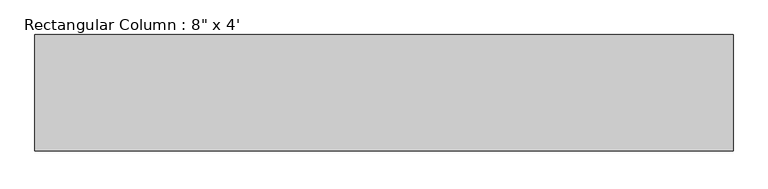
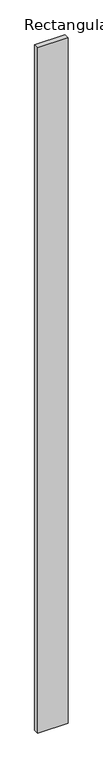
"""IFC4 building model written with IfcOpenShell, lengths in millimetres: column geometry."""

from ifc_helpers import new_model, si_unit, origin, origin_with_axes, place, context, project, spatial, polyline, outline, extrude, source, transform, mapped, element, save


def column_a28f250a(model_context):
    return source(origin(), model_context, "Body", "SweptSolid", [
        extrude(outline(polyline([(609.6, 101.6), (609.6, -101.6), (-609.6, -101.6), (-609.6, 101.6), (609.6, 101.6)])), origin_with_axes(), (0.0, 0.0, 1.0), 29108.4),
    ])


if __name__ == "__main__":
    model = new_model("IFC4")
    model_context = context("Model", 3, world=origin())
    ifc_project = project(units=[si_unit("LENGTHUNIT", "METRE", prefix="MILLI")], contexts=[model_context])
    site = spatial("IfcSite", under=ifc_project)
    building = spatial("IfcBuilding", under=site)
    placement = place(None, origin())
    column_shape = column_a28f250a(model_context)
    element("IfcColumn", 1, ObjectType="Rectangular Column : 8\" x 4'", at=placement, inside=building, context=model_context, shape_type="MappedRepresentation", body=[
        mapped(column_shape, transform((0.0, 0.0, 0.0), x_axis=(1.0, 0.0, 0.0), y_axis=(0.0, 1.0, 0.0), z_axis=(0.0, 0.0, 1.0))),
    ])
    save(model, "model.ifc")

# Revit data of these elements
# Type "Rectangular Column : 8\" x 4'"
#   Assembly Code = "B1010200"
#   Depth = 0' - 8"
#   Offset Base = 0' - 0"
#   Offset Top = 0' - 0"
#   Width = 4' - 0"
#   Material = none
